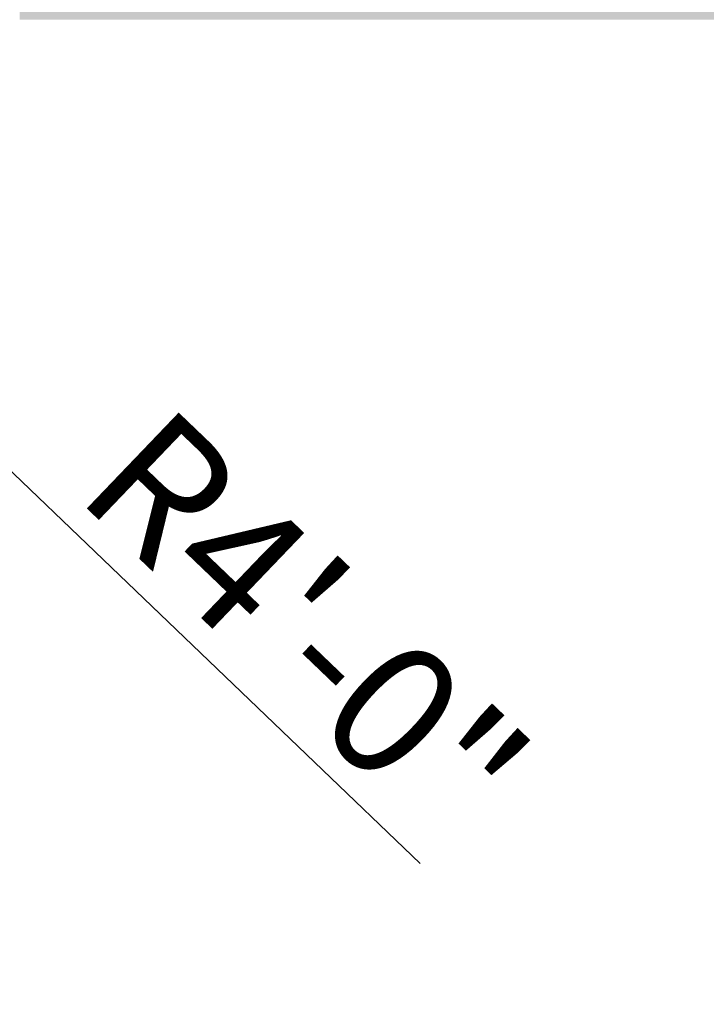
# Model space of a CAD drawing. Units: inches. Extents: x 2083 to 3317, y 1141 to 2115.
# Tile 121 of 256: x 2944 to 3006, y 1327 to 1416. Entities that reach past the tile are written whole.
import ezdxf

# ---------------------------------------------------------------- set-up
doc = ezdxf.new("R2010")
doc.units = ezdxf.units.IN
doc.layers.add('A-ANNO-DIMS', color=2, linetype='Continuous', lineweight=18)
doc.layers.add('A-WALL-PATT', color=251, linetype='Continuous', lineweight=13, true_color=0x636466)
doc.styles.get("Standard").update_dxf_attribs({"font": 'arial.ttf'})
doc.dimstyles.new('ISO-25', dxfattribs={"dimtxt": 12, "dimasz": 12, "dimexe": 1.25, "dimexo": 0.625, "dimtad": 1, "dimlunit": 3, "dimtxsty": 'Standard', "dimcen": 2.5, "dimadec": 0, "dimazin": 0, "dimtfac": 1, "dimtmove": 0, "dimatfit": 3, "dimfxl": 1, "dimarcsym": 0})

# ---------------------------------------------------------------- blocks, each defined once
blk = doc.blocks.new('*D73')
at = {"layer": 'A-ANNO-DIMS', "color": 0, "lineweight": -2, "transparency": 16777216}
for p, q in [((2895.865, 1420.763), (2930.553, 1387.52)), ((2980.105, 1340.032), (2939.217, 1379.217))]:
    blk.add_line(p, q, dxfattribs=at)
at = {"layer": 'A-ANNO-DIMS', "color": 0, "transparency": 16777216}
blk.add_solid([(2940.601, 1380.661), (2937.833, 1377.773), (2930.553, 1387.52)], dxfattribs=at)
at = {"layer": 'Defpoints', "color": 0, "transparency": 16777216}
for p in [(2895.865, 1420.763), (2930.553, 1387.52)]:
    blk.add_point(p, dxfattribs=at)
at = {"layer": 'A-ANNO-DIMS', "color": 0, "transparency": 16777216, "insert": (2968.665, 1360.348), "char_height": 12, "attachment_point": 5, "rotation": 316.21871}
blk.add_mtext('R4\'-0"', dxfattribs=at)

msp = doc.modelspace()

# ---------------------------------------------------------------- hatches: boundary and pattern name
at = {"layer": 'A-WALL-PATT'}
h = msp.add_hatch(color=256, dxfattribs=at)
h.dxf.hatch_style = 1
h.paths.add_polyline_path([(3126.96, 2020.761), (2748.96, 2020.761), (2604.96, 2020.761), (2226.96, 2020.761), (2226.96, 1702.761), (2466.96, 1702.761), (2466.96, 1582.761), (2418.96, 1582.761), (2418.96, 1477.761), (2226.96, 1477.761), (2226.96, 1263.261), (2544.96, 1263.261), (2544.96, 1411.761), (2604.96, 1411.761), (2685.96, 1411.761), (2685.96, 1420.761), (2604.96, 1420.761), (2604.96, 1573.761), (2604.96, 1702.761), (2604.96, 2011.761), (2748.96, 2011.761), (2748.96, 1702.761), (2862.96, 1702.761), (2862.96, 1621.761), (2871.96, 1621.761), (2871.96, 1702.761), (2883.96, 1702.761), (2883.96, 1706.939, -0.026459), (2883.96, 1711.761), (2757.96, 1711.761), (2757.96, 1807.761), (2787.96, 1807.761), (2787.96, 1812.261), (2757.96, 1812.261), (2757.96, 2011.761), (2877.96, 2011.761), (2877.96, 1812.261), (2847.96, 1812.261), (2847.96, 1807.761), (2889.836, 1807.761), (2889.836, 1812.261), (2882.46, 1812.261), (2882.46, 2011.761), (3117.96, 2011.761), (3117.96, 1812.261), (2937.836, 1812.261), (2937.836, 1807.761), (2995.71, 1807.761), (2995.71, 1796.118), (3000.21, 1796.118), (3000.21, 1807.761), (3117.96, 1807.761), (3117.96, 1711.761), (3000.21, 1711.761), (3000.21, 1760.118), (2998.573, 1760.118, -0.020711), (2995.71, 1760.118), (2995.71, 1711.761), (2931.96, 1711.761), (2931.96, 1702.761), (3126.96, 1702.761)])
h.paths.add_polyline_path([(2471.46, 2011.761), (2471.46, 1810.011), (2462.717, 1810.011), (2462.717, 1805.511), (2505.96, 1805.511), (2505.96, 1810.011), (2475.96, 1810.011), (2475.96, 2011.761), (2595.96, 2011.761), (2595.96, 1810.011), (2565.96, 1810.011), (2565.96, 1805.511), (2595.96, 1805.511), (2595.96, 1711.761), (2235.96, 1711.761), (2235.96, 1805.511), (2353.71, 1805.511), (2353.71, 1796.054), (2358.21, 1796.054), (2358.21, 1805.511), (2414.717, 1805.511), (2414.717, 1810.011), (2235.96, 1810.011), (2235.96, 2011.761)], flags=16)
h.paths.add_polyline_path([(2270.205, 1994.61), (2270.205, 1970.61), (2246.205, 1970.61), (2246.205, 1994.61)], flags=0)
edge = h.paths.add_edge_path(flags=0)
edge.add_ellipse((2332.027, 1899.798), major_axis=(-3.043, 3.043), ratio=0.168252, start_angle=-161.33217, end_angle=-156.30711, ccw=False)
edge.add_ellipse((2333.082, 1898.744), major_axis=(-1.055, 1.055), ratio=0.453532, start_angle=-123.37102, end_angle=-94.15911)
edge = h.paths.add_edge_path(flags=0)
edge.add_ellipse((2332.027, 1968.876), major_axis=(3.043, 3.043), ratio=0.168252, start_angle=18.66783, end_angle=23.69289)
edge.add_spline(control_points=[(2332.926, 1970.691), (2332.227, 1970.336), (2330.894, 1969.659), (2328.413, 1970.932), (2327.204, 1967.749), (2324.71, 1969.956), (2322.533, 1967.012), (2320.013, 1971.296), (2317.68, 1968.158), (2316.041, 1967.102), (2315.427, 1966.81)], knot_values=[0, 0, 0, 0, 2.267059, 4.324559, 6.685584, 8.878641, 11.121502, 14.300359, 17.755284, 19.732645, 19.732645, 19.732645, 19.732645], degree=3, periodic=0)
edge.add_ellipse((2332.027, 1968.876), major_axis=(3.043, 3.043), ratio=0.168252, start_angle=18.66783, end_angle=23.69289, ccw=False)
edge.add_ellipse((2333.082, 1969.931), major_axis=(1.055, 1.055), ratio=0.453532, start_angle=56.62898, end_angle=85.84089, ccw=False)
edge = h.paths.add_edge_path(flags=0)
edge.add_spline(control_points=[(2296.428, 1967.988), (2293.628, 1965.336), (2287.704, 1959.727), (2299.744, 1949.996), (2294.533, 1935.669), (2290.573, 1920.604), (2293.394, 1909.974), (2296.185, 1904.967)], knot_values=[0.099185, 0.099185, 0.099185, 0.099185, 0.345301, 0.619822, 0.982653, 1.386093, 1.810555, 1.810555, 1.810555, 1.810555], degree=3, periodic=0)
edge.add_spline(control_points=[(2296.185, 1904.967), (2297.384, 1902.619), (2298.001, 1901.949), (2298.553, 1901.468)], knot_values=[0.006246, 0.006246, 0.006246, 0.006246, 0.055476, 0.055476, 0.055476, 0.055476], degree=3, periodic=0)
edge.add_spline(control_points=[(2298.553, 1901.468), (2297.259, 1900.923), (2295.225, 1900.232), (2293.06, 1900.614), (2292.101, 1900.788), (2292.09, 1900.791)], knot_values=[0.312835, 0.312835, 0.312835, 0.312835, 0.40178, 0.474987, 0.475903, 0.475903, 0.475903, 0.475903], degree=3, periodic=0)
edge.add_arc((2292.794, 1904.664), 3.937, 215.4209, 259.69818, ccw=False)
edge.add_spline(control_points=[(2289.585, 1902.382), (2289.477, 1902.535), (2289.368, 1902.688), (2289.261, 1902.841)], knot_values=[0.102872, 0.102872, 0.102872, 0.102872, 0.116896, 0.116896, 0.116896, 0.116896], degree=3, periodic=0)
edge.add_spline(control_points=[(2289.261, 1902.841), (2288.687, 1902.55), (2287.64, 1902.02), (2285.881, 1901.874), (2283.853, 1901.504), (2281.72, 1899.711), (2278.467, 1899.493), (2276.157, 1901.883), (2272.259, 1899.804), (2267.778, 1901.843), (2262.244, 1900.184), (2257.415, 1901.782), (2254.318, 1900.726), (2253.178, 1900.337)], knot_values=[0, 0, 0, 0, 1.907977, 3.477176, 5.261074, 7.972851, 11.680248, 13.717921, 16.939592, 22.789562, 27.502503, 33.595215, 37.145618, 37.145618, 37.145618, 37.145618], degree=3, periodic=0)
edge.add_line((2253.178, 1900.337), (2250.244, 1902.841))
edge.add_line((2250.244, 1902.841), (2250.244, 1965.833))
edge.add_line((2250.244, 1965.833), (2253.178, 1968.337))
edge.add_spline(control_points=[(2253.178, 1968.337), (2254.318, 1967.948), (2257.415, 1966.892), (2262.244, 1968.49), (2267.778, 1966.831), (2271.527, 1968.537), (2273.876, 1967.828), (2274.207, 1967.728)], knot_values=[0, 0, 0, 0, 0.09018, 0.244935, 0.364644, 0.513233, 0.537855, 0.537855, 0.537855, 0.537855], degree=3, periodic=0)
edge.add_arc((2274.353, 1963.793), 3.937, 72.05113, 92.12795, ccw=False)
edge.add_arc((2281.297, 1985.23), 18.596, 252.05113, 288.56572)
edge.add_arc((2292.317, 1956.029), 12.646, 71.02679, 113.77822, ccw=False)
edge = h.paths.add_edge_path(flags=0)
edge.add_spline(control_points=[(2274.899, 1951.856), (2275.066, 1951.617), (2275.233, 1951.377), (2275.398, 1951.136)], knot_values=[1.409916, 1.409916, 1.409916, 1.409916, 1.43159, 1.43159, 1.43159, 1.43159], degree=3, periodic=0)
edge.add_spline(control_points=[(2275.398, 1951.136), (2275.792, 1950.562), (2276.179, 1949.984), (2276.546, 1949.397)], knot_values=[1.358238, 1.358238, 1.358238, 1.358238, 1.409916, 1.409916, 1.409916, 1.409916], degree=3, periodic=0)
edge.add_line((2276.546, 1949.397), (2277.437, 1947.862))
edge.add_spline(control_points=[(2277.437, 1947.862), (2276.304, 1945.673), (2274.64, 1942.427), (2274.632, 1938.094), (2272.799, 1930.852), (2274.356, 1943.897), (2275.948, 1947.923), (2276.546, 1949.397)], knot_values=[0.005632, 0.005632, 0.005632, 0.005632, 0.186014, 0.266002, 0.357087, 0.59639, 0.739732, 0.739732, 0.739732, 0.739732], degree=3, periodic=0)
edge.add_spline(control_points=[(2276.546, 1949.397), (2276.179, 1949.984), (2275.792, 1950.562), (2275.398, 1951.136)], knot_values=[1.358238, 1.358238, 1.358238, 1.358238, 1.409916, 1.409916, 1.409916, 1.409916], degree=3, periodic=0)
edge.add_spline(control_points=[(2275.398, 1951.136), (2274.943, 1950.08), (2274.208, 1948.025), (2273.935, 1944.851), (2272.469, 1937.627), (2273.466, 1945.696), (2274.701, 1951.059), (2274.899, 1951.856)], knot_values=[0.104364, 0.104364, 0.104364, 0.104364, 0.189636, 0.269624, 0.36071, 0.600013, 0.644622, 0.644622, 0.644622, 0.644622], degree=3, periodic=0)
h.paths.add_polyline_path([(2269.168, 1963.128, -0.357527), (2268.171, 1960.976, -0.092561), (2268.171, 1939.436, -0.357527), (2269.168, 1937.285, -0.357527), (2267.016, 1938.282, -0.164785), (2254.686, 1938.282, -0.357527), (2252.534, 1937.285, -0.357527), (2253.531, 1939.436, -0.092561), (2253.531, 1960.976, -0.357527), (2252.534, 1963.128, -0.357527), (2254.686, 1962.131, -0.164785), (2267.016, 1962.131, -0.357527)], flags=0)
h.paths.add_polyline_path([(2248.874, 1967.802), (2248.874, 1957.028), (2249.458, 1957.028), (2249.458, 1911.647), (2248.874, 1911.647), (2248.874, 1900.873), (2246.512, 1900.873, 0.197327), (2244.15, 1902.457), (2244.15, 1966.218, 0.197327), (2246.512, 1967.802)], flags=0)
h.paths.add_polyline_path([(2269.168, 1931.389, -0.357527), (2268.171, 1929.238, -0.092561), (2268.171, 1907.698, -0.357527), (2269.168, 1905.547, -0.357527), (2267.016, 1906.544, -0.164785), (2254.686, 1906.544, -0.357527), (2252.534, 1905.547, -0.357527), (2253.531, 1907.698, -0.092561), (2253.531, 1929.238, -0.357527), (2252.534, 1931.389, -0.357527), (2254.686, 1930.392, -0.164785), (2267.016, 1930.392, -0.357527)], flags=0)
edge = h.paths.add_edge_path(flags=0)
edge.add_spline(control_points=[(2276.197, 1906.724), (2276.168, 1909.029), (2276.114, 1913.372), (2270.598, 1924.925), (2273.905, 1919.013), (2275.922, 1916.262), (2275.475, 1912.402), (2277.258, 1910.381), (2276.696, 1908.225), (2276.646, 1906.813), (2276.618, 1906.008)], knot_values=[0, 0, 0, 0, 8.61026, 16.221274, 18.843057, 23.804898, 27.440828, 29.356102, 31.203478, 33.650687, 33.650687, 33.650687, 33.650687], degree=3, periodic=0)
edge.add_spline(control_points=[(2276.618, 1906.008), (2276.623, 1905.624), (2276.498, 1904.629), (2275.442, 1903.855), (2274.937, 1903.08), (2274.859, 1902.841)], knot_values=[0.156488, 0.156488, 0.156488, 0.156488, 0.184398, 0.231376, 0.250598, 0.250598, 0.250598, 0.250598], degree=3, periodic=0)
edge.add_line((2274.859, 1902.841), (2276.506, 1902.841))
edge.add_spline(control_points=[(2276.506, 1902.841), (2276.788, 1903.085), (2277.665, 1904.125), (2278.25, 1904.341), (2277.654, 1908.527), (2278.156, 1906.228), (2278.1, 1905.286), (2278.847, 1904.069), (2277.857, 1903.415), (2277.874, 1902.991), (2277.904, 1902.841)], knot_values=[0.059574, 0.059574, 0.059574, 0.059574, 0.080753, 0.103741, 0.16972, 0.176036, 0.207137, 0.240474, 0.262341, 0.27366, 0.27366, 0.27366, 0.27366], degree=3, periodic=0)
edge.add_line((2277.904, 1902.841), (2280.03, 1902.841))
edge.add_spline(control_points=[(2280.03, 1902.841), (2279.888, 1903.088), (2279.499, 1903.982), (2280.152, 1905.939), (2278.104, 1909.658), (2279.762, 1907.185), (2280.328, 1904.875), (2280.485, 1903.49), (2281.463, 1903.249), (2281.758, 1902.936), (2281.834, 1902.841)], knot_values=[0.013856, 0.013856, 0.013856, 0.013856, 0.034874, 0.088867, 0.107879, 0.126738, 0.158714, 0.193757, 0.217487, 0.226722, 0.226722, 0.226722, 0.226722], degree=3, periodic=0)
edge.add_spline(control_points=[(2281.834, 1902.841), (2281.788, 1902.827), (2281.647, 1902.783), (2281.396, 1902.859), (2281.088, 1902.985), (2280.721, 1903.061), (2280.333, 1903.026), (2280.125, 1902.899), (2280.03, 1902.841)], knot_values=[0, 0, 0, 0, 0.14413, 0.435517, 0.749276, 1.153046, 1.548371, 1.878348, 1.878348, 1.878348, 1.878348], degree=3, periodic=0)
edge.add_line((2280.03, 1902.841), (2277.904, 1902.841))
edge.add_spline(control_points=[(2277.904, 1902.841), (2277.893, 1902.796), (2277.865, 1902.68), (2277.607, 1902.687), (2277.274, 1902.801), (2276.838, 1902.62), (2276.584, 1902.789), (2276.506, 1902.841)], knot_values=[0, 0, 0, 0, 0.127189, 0.326199, 0.628009, 1.24357, 1.515331, 1.515331, 1.515331, 1.515331], degree=3, periodic=0)
edge.add_line((2276.506, 1902.841), (2274.859, 1902.841))
edge.add_spline(control_points=[(2274.859, 1902.841), (2274.814, 1902.899), (2274.725, 1903.013), (2274.493, 1903.119), (2274.244, 1902.961), (2273.937, 1903.185), (2273.614, 1902.983), (2273.408, 1902.883), (2273.322, 1902.841)], knot_values=[0, 0, 0, 0, 0.21843, 0.436957, 0.687977, 0.990379, 1.398396, 1.69185, 1.69185, 1.69185, 1.69185], degree=3, periodic=0)
edge.add_spline(control_points=[(2273.322, 1902.841), (2273.617, 1903.446), (2274.274, 1904.538), (2276.027, 1904.574), (2276.207, 1906.584), (2276.197, 1906.724)], knot_values=[0.012227, 0.012227, 0.012227, 0.012227, 0.059472, 0.106218, 0.134458, 0.134458, 0.134458, 0.134458], degree=3, periodic=0)
h.paths.add_polyline_path([(2270.776, 1897.79), (2270.776, 1873.79), (2246.776, 1873.79), (2246.776, 1897.79)], flags=0)
h.paths.add_polyline_path([(2353.71, 1760.005), (2353.71, 1760.054), (2358.21, 1760.054, -0.033729)], flags=0)
h.paths.add_polyline_path([(2321.819, 1737.529), (2341.995, 1737.529, -0.414214), (2343.203, 1736.321), (2343.203, 1721.021, -0.414214), (2341.995, 1719.813), (2321.819, 1719.813, -0.414214), (2320.611, 1721.021), (2320.611, 1736.321, -0.414214)], flags=0)
h.paths.add_polyline_path([(2324.235, 1736.321), (2339.579, 1736.321, -0.414214), (2341.995, 1733.905), (2341.995, 1725.45, -0.414214), (2339.579, 1723.034), (2333.681, 1723.034), (2333.845, 1722.045, -0.870646), (2335.425, 1721.826, -0.767327), (2333.923, 1721.423), (2331.291, 1721.423, -0.767327), (2329.788, 1721.826, -0.870646), (2331.368, 1722.045), (2331.533, 1723.034), (2324.235, 1723.034, -0.414214), (2321.819, 1725.45), (2321.819, 1733.905, -0.414214)], flags=0)
h.paths.add_polyline_path([(2570.484, 1928.615), (2589.684, 1928.615), (2590.169, 1928.615), (2590.169, 1904.993), (2570.484, 1904.993)], flags=0)
h.paths.add_polyline_path([(2574.447, 1927.264, -1), (2572.829, 1927.264, -1)], flags=0)
h.paths.add_polyline_path([(2573.09, 1926.941), (2573.925, 1927.776), (2574.148, 1927.553), (2573.313, 1926.718)], flags=0)
h.paths.add_polyline_path([(2578.779, 1919.73, -1), (2571.592, 1919.73, -1)], flags=0)
h.paths.add_polyline_path([(2578.385, 1919.73, -1), (2571.985, 1919.73, -1)], flags=0)
h.paths.add_polyline_path([(2331.596, 1729.476, -1), (2333.618, 1729.476, -1)], flags=0)
h.paths.add_polyline_path([(2578.034, 1927.264, -1), (2576.416, 1927.264, -1)], flags=0)
h.paths.add_polyline_path([(2576.689, 1927.531), (2576.912, 1927.754), (2577.747, 1926.919), (2577.524, 1926.696)], flags=0)
h.paths.add_polyline_path([(2578.139, 1909.86, -1), (2572.232, 1909.86, -1)], flags=0)
h.paths.add_polyline_path([(2577.745, 1909.86, -1), (2572.625, 1909.86, -1)], flags=0)
h.paths.add_polyline_path([(2583.798, 1927.264, -1), (2582.179, 1927.264, -1)], flags=0)
h.paths.add_polyline_path([(2582.719, 1927.754), (2583.554, 1926.919), (2583.331, 1926.696), (2582.496, 1927.531)], flags=0)
h.paths.add_polyline_path([(2582.496, 1927.531), (2582.719, 1927.754), (2583.554, 1926.919), (2583.331, 1926.696)], flags=0)
h.paths.add_polyline_path([(2587.739, 1920.53, -1), (2581.832, 1920.53, -1)], flags=0)
h.paths.add_polyline_path([(2587.345, 1920.53, -1), (2582.225, 1920.53, -1)], flags=0)
h.paths.add_polyline_path([(2587.385, 1927.264, -1), (2585.766, 1927.264, -1)], flags=0)
h.paths.add_polyline_path([(2586.082, 1926.98), (2586.917, 1927.815), (2587.14, 1927.593), (2586.305, 1926.758)], flags=0)
h.paths.add_polyline_path([(2588.379, 1910.66, -1), (2581.192, 1910.66, -1)], flags=0)
h.paths.add_polyline_path([(2587.985, 1910.66, -1), (2581.585, 1910.66, -1)], flags=0)
h.paths.add_polyline_path([(2417.168, 1729.478), (2437.344, 1729.478, -0.414214), (2438.552, 1728.27), (2438.552, 1712.969, -0.414214), (2437.344, 1711.761), (2417.168, 1711.761, -0.414214), (2415.96, 1712.969), (2415.96, 1728.27, -0.414214)], flags=0)
h.paths.add_polyline_path([(2419.584, 1728.27), (2434.928, 1728.27, -0.414214), (2437.344, 1725.854), (2437.344, 1717.398, -0.414214), (2434.928, 1714.983), (2429.029, 1714.983), (2429.194, 1713.994, -0.870646), (2430.774, 1713.775, -0.767327), (2429.271, 1713.372), (2426.64, 1713.372, -0.767327), (2425.137, 1713.775, -0.870646), (2426.717, 1713.994), (2426.882, 1714.983), (2419.584, 1714.983, -0.414214), (2417.168, 1717.398), (2417.168, 1725.854, -0.414214)], flags=0)
h.paths.add_polyline_path([(2419.584, 1728.27), (2434.928, 1728.27, -0.414214), (2437.344, 1725.854), (2437.344, 1717.398, -0.414214), (2434.928, 1714.983), (2429.029, 1714.983), (2428.358, 1719.009), (2427.553, 1719.009), (2426.882, 1714.983), (2419.584, 1714.983, -0.414214), (2417.168, 1717.398), (2417.168, 1725.854, -0.414214)], flags=0)
h.paths.add_polyline_path([(2426.944, 1721.425, -1), (2428.967, 1721.425, -1)], flags=0)
h.paths.add_polyline_path([(2475.96, 1702.761), (2595.96, 1702.761), (2595.96, 1582.761), (2475.96, 1582.761)], flags=16)
h.paths.add_polyline_path([(2427.96, 1573.761), (2595.96, 1573.761), (2595.96, 1468.761), (2595.96, 1420.761), (2384.46, 1420.761), (2384.46, 1468.761), (2427.96, 1468.761)], flags=16)
h.paths.add_polyline_path([(2379.96, 1468.761), (2379.96, 1420.761), (2235.96, 1420.761), (2235.96, 1468.761)], flags=16)
h.paths.add_polyline_path([(2317.816, 1466.696), (2337.992, 1466.696, -0.414214), (2339.2, 1465.488), (2339.2, 1450.187, -0.414214), (2337.992, 1448.979), (2317.816, 1448.979, -0.414214), (2316.608, 1450.187), (2316.608, 1465.488, -0.414214)], flags=0)
h.paths.add_polyline_path([(2320.232, 1465.488), (2335.576, 1465.488, -0.414214), (2337.992, 1463.072), (2337.992, 1454.616, -0.414214), (2335.576, 1452.2), (2329.677, 1452.2), (2329.842, 1451.212, -0.870646), (2331.422, 1450.992, -0.767327), (2329.92, 1450.59), (2327.288, 1450.59, -0.767327), (2325.785, 1450.992, -0.870646), (2327.365, 1451.212), (2327.53, 1452.2), (2320.232, 1452.2, -0.414214), (2317.816, 1454.616), (2317.816, 1463.072, -0.414214)], flags=0)
h.paths.add_polyline_path([(2320.232, 1465.488), (2335.576, 1465.488, -0.414214), (2337.992, 1463.072), (2337.992, 1454.616, -0.414214), (2335.576, 1452.2), (2329.677, 1452.2), (2329.006, 1456.227), (2328.201, 1456.227), (2327.53, 1452.2), (2320.232, 1452.2, -0.414214), (2317.816, 1454.616), (2317.816, 1463.072, -0.414214)], flags=0)
h.paths.add_polyline_path([(2327.593, 1458.643, -1), (2329.615, 1458.643, -1)], flags=0)
h.paths.add_polyline_path([(2244.412, 1433.34), (2241.921, 1433.34, -0.414214), (2240.018, 1435.244), (2240.018, 1440.953, -0.414211), (2241.921, 1442.856), (2244.412, 1442.856, -1.976472)], flags=0)
h.paths.add_polyline_path([(2245.357, 1434.398, -0.414214), (2245.357, 1441.799, -2.144098)], flags=0)
h.paths.add_polyline_path([(2535.96, 1416.261), (2535.96, 1272.261), (2235.96, 1272.261), (2235.96, 1416.261)], flags=16)
h.paths.add_polyline_path([(2260.12, 1384.293), (2260.12, 1362.039), (2237.865, 1362.039), (2237.865, 1384.293)], flags=0)
edge = h.paths.add_edge_path(flags=0)
edge.add_line((2318.252, 1362.093), (2318.146, 1362.001))
edge.add_ellipse((2317.445, 1360.431), major_axis=(2.822, 2.822), ratio=0.168252, start_angle=18.66783, end_angle=20.94813, ccw=False)
edge.add_ellipse((2318.423, 1361.409), major_axis=(0.978, 0.978), ratio=0.453532, start_angle=56.62898, end_angle=70.2262, ccw=False)
edge = h.paths.add_edge_path(flags=0)
edge.add_line((2319.107, 1295.571), (2319.015, 1295.677))
edge.add_ellipse((2317.445, 1296.378), major_axis=(-2.822, 2.822), ratio=0.168252, start_angle=-161.33217, end_angle=-159.05187, ccw=False)
edge.add_ellipse((2318.423, 1295.4), major_axis=(-0.978, 0.978), ratio=0.453532, start_angle=-123.37102, end_angle=-109.7738)
edge = h.paths.add_edge_path(flags=0)
edge.add_spline(control_points=[(2284.21, 1301.17), (2284.581, 1300.445), (2284.891, 1299.892), (2285.16, 1299.461)], knot_values=[0.039066, 0.039066, 0.039066, 0.039066, 0.055476, 0.055476, 0.055476, 0.055476], degree=3, periodic=0)
edge.add_line((2285.16, 1299.461), (2284.21, 1301.17))
edge = h.paths.add_edge_path(flags=0)
edge.add_line((2280.412, 1297.298), (2283.37, 1297.036))
edge.add_line((2283.37, 1297.036), (2286.406, 1297.926))
edge.add_spline(control_points=[(2286.406, 1297.926), (2285.305, 1297.463), (2284.345, 1297.129), (2283.37, 1297.036)], knot_values=[0.394369, 0.394369, 0.394369, 0.394369, 0.475903, 0.475903, 0.475903, 0.475903], degree=3, periodic=0)
edge.add_spline(control_points=[(2283.37, 1297.036), (2283.281, 1297.028), (2282.316, 1296.957), (2281.313, 1297.134), (2280.423, 1297.296), (2280.412, 1297.298)], knot_values=[0.312835, 0.312835, 0.312835, 0.312835, 0.320246, 0.393453, 0.394369, 0.394369, 0.394369, 0.394369], degree=3, periodic=0)
edge = h.paths.add_edge_path(flags=0)
edge.add_line((2284.436, 1359.607), (2280.446, 1355.328))
edge.add_line((2280.446, 1355.328), (2279.58, 1351.018))
edge.add_line((2279.58, 1351.018), (2282.413, 1346.58))
edge.add_spline(control_points=[(2282.413, 1346.58), (2283.153, 1345.589), (2284.253, 1344.029), (2284.801, 1342.387), (2284.935, 1341.806)], knot_values=[1.240098, 1.240098, 1.240098, 1.240098, 1.332892, 1.382712, 1.382712, 1.382712, 1.382712], degree=3, periodic=0)
edge.add_spline(control_points=[(2284.935, 1341.806), (2285.319, 1340.141), (2285.233, 1338.409), (2284.91, 1336.654)], knot_values=[1.097484, 1.097484, 1.097484, 1.097484, 1.240098, 1.240098, 1.240098, 1.240098], degree=3, periodic=0)
edge.add_spline(control_points=[(2284.91, 1336.654), (2284.587, 1334.899), (2284.027, 1333.12), (2283.463, 1331.361)], knot_values=[0.95487, 0.95487, 0.95487, 0.95487, 1.097484, 1.097484, 1.097484, 1.097484], degree=3, periodic=0)
edge.add_line((2283.463, 1331.361), (2281.89, 1326.153))
edge.add_line((2281.89, 1326.153), (2280.756, 1321.056))
edge.add_line((2280.756, 1321.056), (2280.299, 1316.002))
edge.add_line((2280.299, 1316.002), (2280.716, 1310.95))
edge.add_line((2280.716, 1310.95), (2282.028, 1305.972))
edge.add_line((2282.028, 1305.972), (2284.21, 1301.17))
edge.add_spline(control_points=[(2284.21, 1301.17), (2283.341, 1302.73), (2282.612, 1304.336), (2282.028, 1305.972)], knot_values=[0.099185, 0.099185, 0.099185, 0.099185, 0.241799, 0.241799, 0.241799, 0.241799], degree=3, periodic=0)
edge.add_spline(control_points=[(2282.028, 1305.972), (2281.444, 1307.608), (2281.005, 1309.273), (2280.716, 1310.95)], knot_values=[0.241799, 0.241799, 0.241799, 0.241799, 0.384413, 0.384413, 0.384413, 0.384413], degree=3, periodic=0)
edge.add_spline(control_points=[(2280.716, 1310.95), (2280.433, 1312.588), (2280.289, 1314.277), (2280.299, 1315.962), (2280.299, 1316.002)], knot_values=[0.384413, 0.384413, 0.384413, 0.384413, 0.523647, 0.527028, 0.527028, 0.527028, 0.527028], degree=3, periodic=0)
edge.add_spline(control_points=[(2280.299, 1316.002), (2280.312, 1317.687), (2280.478, 1319.368), (2280.756, 1321.056)], knot_values=[0.527028, 0.527028, 0.527028, 0.527028, 0.669642, 0.669642, 0.669642, 0.669642], degree=3, periodic=0)
edge.add_spline(control_points=[(2280.756, 1321.056), (2281.035, 1322.744), (2281.426, 1324.44), (2281.89, 1326.153)], knot_values=[0.669642, 0.669642, 0.669642, 0.669642, 0.812256, 0.812256, 0.812256, 0.812256], degree=3, periodic=0)
edge.add_spline(control_points=[(2281.89, 1326.153), (2282.264, 1327.533), (2282.788, 1329.262), (2283.353, 1331.018), (2283.463, 1331.361)], knot_values=[0.812256, 0.812256, 0.812256, 0.812256, 0.927087, 0.95487, 0.95487, 0.95487, 0.95487], degree=3, periodic=0)
edge.add_line((2283.463, 1331.361), (2284.91, 1336.654))
edge.add_line((2284.91, 1336.654), (2284.935, 1341.806))
edge.add_line((2284.935, 1341.806), (2282.413, 1346.58))
edge.add_spline(control_points=[(2282.413, 1346.58), (2281.275, 1348.104), (2280.078, 1349.57), (2279.58, 1351.018)], knot_values=[1.382712, 1.382712, 1.382712, 1.382712, 1.525326, 1.525326, 1.525326, 1.525326], degree=3, periodic=0)
edge.add_spline(control_points=[(2279.58, 1351.018), (2279.443, 1351.415), (2279.136, 1352.857), (2279.735, 1354.29), (2280.446, 1355.328)], knot_values=[1.525326, 1.525326, 1.525326, 1.525326, 1.564439, 1.667941, 1.667941, 1.667941, 1.667941], degree=3, periodic=0)
edge.add_spline(control_points=[(2280.446, 1355.328), (2281.426, 1356.758), (2282.931, 1358.183), (2284.436, 1359.607)], knot_values=[1.667941, 1.667941, 1.667941, 1.667941, 1.810555, 1.810555, 1.810555, 1.810555], degree=3, periodic=0)
edge.add_arc((2280.623, 1348.518), 11.726, 71.02679, 113.77822)
edge.add_arc((2270.405, 1375.595), 17.244, 252.05113, 288.56572, ccw=False)
edge.add_arc((2263.966, 1355.718), 3.651, 72.05113, 92.12795)
edge.add_arc((2263.966, 1355.718), 3.651, 92.12795, 177.98513)
edge.add_spline(control_points=[(2260.318, 1355.846), (2260.26, 1354.221), (2260.551, 1350.187), (2262.999, 1346.766), (2264.473, 1344.649)], knot_values=[1.43159, 1.43159, 1.43159, 1.43159, 1.564144, 1.770695, 1.770695, 1.770695, 1.770695], degree=3, periodic=0)
edge.add_line((2264.473, 1344.649), (2264.936, 1343.983))
edge.add_spline(control_points=[(2263.801, 1340.248), (2263.843, 1340.514), (2264.067, 1341.756), (2264.513, 1343.002), (2264.935, 1343.981)], knot_values=[0.53657, 0.53657, 0.53657, 0.53657, 0.559349, 0.644622, 0.644622, 0.644622, 0.644622], degree=3, periodic=0)
edge.add_spline(control_points=[(2264.935, 1343.981), (2265.118, 1343.715), (2265.299, 1343.448), (2265.477, 1343.179)], knot_values=[1.384077, 1.384077, 1.384077, 1.384077, 1.409916, 1.409916, 1.409916, 1.409916], degree=3, periodic=0)
edge.add_spline(control_points=[(2265.477, 1343.179), (2265.655, 1342.911), (2265.829, 1342.641), (2265.999, 1342.369)], knot_values=[1.358238, 1.358238, 1.358238, 1.358238, 1.384077, 1.384077, 1.384077, 1.384077], degree=3, periodic=0)
edge.add_line((2265.999, 1342.369), (2266.826, 1340.946))
edge.add_spline(control_points=[(2266.826, 1340.946), (2268.894, 1337.09), (2271.398, 1325.843), (2270.516, 1310.569), (2275.919, 1301.861), (2277.79, 1299.199)], knot_values=[0.116896, 0.116896, 0.116896, 0.116896, 0.472987, 1.050969, 1.313793, 1.313793, 1.313793, 1.313793], degree=3, periodic=0)
edge.add_spline(control_points=[(2277.79, 1299.199), (2277.839, 1299.128), (2277.889, 1299.057), (2277.94, 1298.987)], knot_values=[0.109884, 0.109884, 0.109884, 0.109884, 0.116896, 0.116896, 0.116896, 0.116896], degree=3, periodic=0)
edge.add_line((2277.94, 1298.987), (2277.789, 1299.199))
edge.add_spline(control_points=[(2277.789, 1299.199), (2277.257, 1298.929), (2276.286, 1298.438), (2275.039, 1298.334), (2274.383, 1298.239), (2274.215, 1298.209)], knot_values=[33.12187, 33.12187, 33.12187, 33.12187, 35.029056, 36.598255, 37.144827, 37.144827, 37.144827, 37.144827], degree=3, periodic=0)
edge.add_line((2274.215, 1298.209), (2273.073, 1297.893))
edge.add_spline(control_points=[(2273.073, 1297.893), (2272.323, 1297.58), (2271.039, 1296.511), (2269.248, 1296.226), (2268.423, 1296.375)], knot_values=[26.532584, 26.532584, 26.532584, 26.532584, 29.198919, 31.839101, 31.839101, 31.839101, 31.839101], degree=3, periodic=0)
edge.add_line((2268.423, 1296.375), (2263.879, 1297.458))
edge.add_spline(control_points=[(2263.879, 1297.458), (2263.556, 1297.359), (2261.86, 1296.839), (2260.239, 1297.282), (2258.933, 1297.516)], knot_values=[15.919551, 15.919551, 15.919551, 15.919551, 16.939592, 21.226067, 21.226067, 21.226067, 21.226067], degree=3, periodic=0)
edge.add_line((2258.933, 1297.516), (2254.055, 1297.329))
edge.add_spline(control_points=[(2254.055, 1297.329), (2253.756, 1297.296), (2252.114, 1297.165), (2250.462, 1297.544), (2249.13, 1297.668)], knot_values=[5.306517, 5.306517, 5.306517, 5.306517, 6.276435, 10.613034, 10.613034, 10.613034, 10.613034], degree=3, periodic=0)
edge.add_line((2249.13, 1297.668), (2244.332, 1296.878))
edge.add_line((2244.332, 1296.878), (2241.611, 1299.199))
edge.add_line((2241.611, 1299.199), (2241.611, 1357.609))
edge.add_line((2241.611, 1357.609), (2244.332, 1359.931))
edge.add_line((2244.332, 1359.931), (2252.729, 1359.543))
edge.add_spline(control_points=[(2252.729, 1359.543), (2252.871, 1359.546), (2253.306, 1359.548), (2253.74, 1359.514), (2254.032, 1359.482)], knot_values=[0.233291, 0.233291, 0.233291, 0.233291, 0.244935, 0.268927, 0.268927, 0.268927, 0.268927], degree=3, periodic=0)
edge.add_line((2254.032, 1359.482), (2259.587, 1359.416))
edge.add_spline(control_points=[(2259.587, 1359.416), (2260.677, 1359.629), (2262.073, 1359.897), (2263.524, 1359.459), (2263.83, 1359.366)], knot_values=[0.422516, 0.422516, 0.422516, 0.422516, 0.513233, 0.537855, 0.537855, 0.537855, 0.537855], degree=3, periodic=0)
edge.add_arc((2263.966, 1355.718), 3.651, 72.05113, 92.12795, ccw=False)
edge.add_arc((2270.405, 1375.595), 17.244, 252.05113, 288.56572)
edge.add_arc((2280.623, 1348.518), 11.726, 71.02679, 113.77822, ccw=False)
h.paths.add_polyline_path([(2240.341, 1359.435), (2240.341, 1349.444), (2240.882, 1349.444), (2240.882, 1307.365), (2240.341, 1307.365), (2240.341, 1297.374), (2238.15, 1297.374, 0.197327), (2235.96, 1298.843), (2235.96, 1357.966, 0.197327), (2238.15, 1359.435)], flags=0)
h.paths.add_polyline_path([(2259.158, 1355.101, -0.357527), (2258.233, 1353.106, -0.092561), (2258.233, 1333.133, -0.357527), (2259.158, 1331.138, -0.357527), (2257.163, 1332.062, -0.164785), (2245.729, 1332.062, -0.357527), (2243.735, 1331.138, -0.357527), (2244.659, 1333.133, -0.092561), (2244.659, 1353.106, -0.357527), (2243.735, 1355.101, -0.357527), (2245.729, 1354.176, -0.164785), (2257.163, 1354.176, -0.357527)], flags=0)
edge = h.paths.add_edge_path(flags=0)
edge.add_line((2265.999, 1342.369), (2266.826, 1340.946))
edge.add_line((2266.826, 1340.946), (2265.308, 1337.814))
edge.add_line((2265.308, 1337.814), (2264.358, 1334.653))
edge.add_line((2264.358, 1334.653), (2264.262, 1333.8))
edge.add_spline(control_points=[(2264.262, 1333.8), (2264.208, 1333.187), (2264.162, 1332.366), (2264.007, 1331.414), (2263.969, 1331.202)], knot_values=[0.464444, 0.464444, 0.464444, 0.464444, 0.516691, 0.531608, 0.531608, 0.531608, 0.531608], degree=3, periodic=0)
edge.add_spline(control_points=[(2263.969, 1331.202), (2263.775, 1330.119), (2263.424, 1328.791), (2263.257, 1328.531), (2263.234, 1328.515)], knot_values=[0.372682, 0.372682, 0.372682, 0.372682, 0.44885, 0.464444, 0.464444, 0.464444, 0.464444], degree=3, periodic=0)
edge.add_spline(control_points=[(2263.234, 1328.515), (2263.096, 1328.42), (2263.131, 1329.301), (2263.275, 1330.616)], knot_values=[0.280919, 0.280919, 0.280919, 0.280919, 0.372682, 0.372682, 0.372682, 0.372682], degree=3, periodic=0)
edge.add_spline(control_points=[(2263.275, 1330.616), (2263.419, 1331.93), (2263.672, 1333.677), (2263.97, 1335.315)], knot_values=[0.189157, 0.189157, 0.189157, 0.189157, 0.280919, 0.280919, 0.280919, 0.280919], degree=3, periodic=0)
edge.add_spline(control_points=[(2263.97, 1335.315), (2264.1, 1336.032), (2264.419, 1337.622), (2264.755, 1338.864), (2264.947, 1339.491)], knot_values=[0.097394, 0.097394, 0.097394, 0.097394, 0.137578, 0.189157, 0.189157, 0.189157, 0.189157], degree=3, periodic=0)
edge.add_spline(control_points=[(2264.947, 1339.491), (2265.29, 1340.606), (2265.644, 1341.494), (2265.999, 1342.369)], knot_values=[0.005632, 0.005632, 0.005632, 0.005632, 0.097394, 0.097394, 0.097394, 0.097394], degree=3, periodic=0)
h.paths.add_polyline_path([(2259.158, 1325.671, -0.357527), (2258.233, 1323.676, -0.092561), (2258.233, 1303.703, -0.357527), (2259.158, 1301.708, -0.357527), (2257.163, 1302.633, -0.164785), (2245.729, 1302.633, -0.357527), (2243.735, 1301.708, -0.357527), (2244.659, 1303.703, -0.092561), (2244.659, 1323.676, -0.357527), (2243.735, 1325.671, -0.357527), (2245.729, 1324.747, -0.164785), (2257.163, 1324.747, -0.357527)], flags=0)
edge = h.paths.add_edge_path(flags=0)
edge.add_spline(control_points=[(2261.709, 1317.311), (2261.679, 1317.418), (2261.762, 1317.389), (2262.491, 1316.09), (2262.962, 1315.301)], knot_values=[14.955861, 14.955861, 14.955861, 14.955861, 16.221274, 18.694826, 18.694826, 18.694826, 18.694826], degree=3, periodic=0)
edge.add_spline(control_points=[(2262.962, 1315.301), (2262.99, 1315.254), (2263.702, 1314.067), (2264.349, 1313.127), (2264.73, 1312.164)], knot_values=[18.694826, 18.694826, 18.694826, 18.694826, 18.843057, 22.433791, 22.433791, 22.433791, 22.433791], degree=3, periodic=0)
edge.add_spline(control_points=[(2264.73, 1312.164), (2264.876, 1311.796), (2265.177, 1310.77), (2265.143, 1309.559), (2265.248, 1308.824)], knot_values=[22.433791, 22.433791, 22.433791, 22.433791, 23.804898, 26.172756, 26.172756, 26.172756, 26.172756], degree=3, periodic=0)
edge.add_line((2265.248, 1308.824), (2265.851, 1307.172))
edge.add_spline(control_points=[(2265.851, 1307.172), (2266.065, 1306.822), (2266.384, 1306.332), (2266.424, 1305.781), (2266.42, 1305.611)], knot_values=[28.062562, 28.062562, 28.062562, 28.062562, 29.356102, 29.911721, 29.911721, 29.911721, 29.911721], degree=3, periodic=0)
edge.add_spline(control_points=[(2266.42, 1305.611), (2266.416, 1305.433), (2266.394, 1305.25), (2266.365, 1305.066)], knot_values=[29.911721, 29.911721, 29.911721, 29.911721, 30.497837, 30.497837, 30.497837, 30.497837], degree=3, periodic=0)
edge.add_line((2266.365, 1305.066), (2266.066, 1302.136))
edge.add_spline(control_points=[(2266.066, 1302.136), (2266.071, 1301.78), (2265.998, 1301.2), (2265.663, 1300.759), (2265.509, 1300.586)], knot_values=[0.156488, 0.156488, 0.156488, 0.156488, 0.184398, 0.203543, 0.203543, 0.203543, 0.203543], degree=3, periodic=0)
edge.add_line((2265.509, 1300.586), (2264.435, 1299.199))
edge.add_line((2264.435, 1299.199), (2265.962, 1299.199))
edge.add_line((2265.962, 1299.199), (2267.336, 1301.175))
edge.add_line((2267.336, 1301.175), (2267.312, 1301.986))
edge.add_spline(control_points=[(2267.312, 1301.986), (2267.261, 1302.862), (2267.16, 1303.737), (2267.271, 1303.326)], knot_values=[0.126229, 0.126229, 0.126229, 0.126229, 0.166617, 0.166617, 0.166617, 0.166617], degree=3, periodic=0)
edge.add_spline(control_points=[(2267.271, 1303.326), (2267.28, 1303.294), (2267.31, 1303.175), (2267.373, 1302.884), (2267.406, 1302.683), (2267.418, 1302.601)], knot_values=[0.166617, 0.166617, 0.166617, 0.166617, 0.16972, 0.176036, 0.180765, 0.180765, 0.180765, 0.180765], degree=3, periodic=0)
edge.add_spline(control_points=[(2267.744, 1300.988), (2267.688, 1301.151), (2267.481, 1301.657), (2267.484, 1302.145), (2267.418, 1302.601)], knot_values=[0.180765, 0.180765, 0.180765, 0.180765, 0.193767, 0.220139, 0.220139, 0.220139, 0.220139], degree=3, periodic=0)
edge.add_line((2267.418, 1302.601), (2267.744, 1300.988))
edge.add_spline(control_points=[(2267.744, 1300.988), (2267.832, 1300.732), (2267.932, 1300.31), (2267.555, 1299.975), (2267.429, 1299.829)], knot_values=[0.220139, 0.220139, 0.220139, 0.220139, 0.240474, 0.25489, 0.25489, 0.25489, 0.25489], degree=3, periodic=0)
edge.add_line((2267.429, 1299.829), (2267.258, 1299.199))
edge.add_line((2267.258, 1299.199), (2269.23, 1299.199))
edge.add_spline(control_points=[(2269.23, 1299.199), (2269.099, 1299.429), (2268.843, 1300.016), (2269.012, 1300.916), (2268.947, 1301.661)], knot_values=[0.013856, 0.013856, 0.013856, 0.013856, 0.034874, 0.067073, 0.067073, 0.067073, 0.067073], degree=3, periodic=0)
edge.add_line((2268.947, 1301.661), (2268.432, 1303.603))
edge.add_spline(control_points=[(2268.432, 1303.603), (2268.176, 1304.192), (2267.596, 1305.251), (2268.041, 1304.623), (2268.251, 1304.282)], knot_values=[0.090155, 0.090155, 0.090155, 0.090155, 0.107879, 0.120289, 0.120289, 0.120289, 0.120289], degree=3, periodic=0)
edge.add_spline(control_points=[(2268.251, 1304.282), (2268.361, 1304.105), (2269.058, 1302.918), (2269.383, 1301.59), (2269.521, 1300.776), (2269.575, 1300.556)], knot_values=[0.120289, 0.120289, 0.120289, 0.120289, 0.126738, 0.158714, 0.173506, 0.173506, 0.173506, 0.173506], degree=3, periodic=0)
edge.add_line((2269.575, 1300.556), (2270.686, 1299.421))
edge.add_spline(control_points=[(2270.686, 1299.421), (2270.767, 1299.357), (2270.838, 1299.281), (2270.903, 1299.199)], knot_values=[0.21816, 0.21816, 0.21816, 0.21816, 0.226722, 0.226722, 0.226722, 0.226722], degree=3, periodic=0)
edge.add_line((2270.937, 1299.193), (2270.903, 1299.199))
edge.add_spline(control_points=[(2270.903, 1299.199), (2270.86, 1299.186), (2270.73, 1299.146), (2270.496, 1299.216), (2270.272, 1299.308), (2270.121, 1299.348), (2270.063, 1299.36)], knot_values=[0.939174, 0.939174, 0.939174, 0.939174, 1.083304, 1.374691, 1.68845, 1.878348, 1.878348, 1.878348, 1.878348], degree=3, periodic=0)
edge.add_line((2270.063, 1299.36), (2269.23, 1299.199))
edge.add_line((2269.23, 1299.199), (2267.258, 1299.199))
edge.add_spline(control_points=[(2267.258, 1299.199), (2267.248, 1299.157), (2267.223, 1299.05), (2266.984, 1299.057), (2266.809, 1299.116), (2266.677, 1299.109), (2266.637, 1299.105)], knot_values=[0.757665, 0.757665, 0.757665, 0.757665, 0.884854, 1.083864, 1.385675, 1.515331, 1.515331, 1.515331, 1.515331], degree=3, periodic=0)
edge.add_spline(control_points=[(2266.637, 1299.105), (2266.485, 1299.089), (2266.236, 1299.017), (2266.035, 1299.151), (2265.962, 1299.199)], knot_values=[0, 0, 0, 0, 0.485905, 0.757665, 0.757665, 0.757665, 0.757665], degree=3, periodic=0)
edge.add_line((2265.962, 1299.199), (2264.435, 1299.199))
edge.add_line((2264.435, 1299.199), (2263.858, 1299.367))
edge.add_spline(control_points=[(2263.858, 1299.367), (2263.819, 1299.371), (2263.78, 1299.386), (2263.74, 1299.402)], knot_values=[0.845925, 0.845925, 0.845925, 0.845925, 0.978627, 0.978627, 0.978627, 0.978627], degree=3, periodic=0)
edge.add_line((2263.722, 1299.396), (2263.01, 1299.199))
edge.add_spline(control_points=[(2263.01, 1299.199), (2263.246, 1299.683), (2263.506, 1300.128), (2263.873, 1300.408)], knot_values=[0.012227, 0.012227, 0.012227, 0.012227, 0.052971, 0.052971, 0.052971, 0.052971], degree=3, periodic=0)
edge.add_spline(control_points=[(2263.873, 1300.408), (2263.932, 1300.453), (2264.084, 1300.553), (2264.255, 1300.624), (2264.36, 1300.665)], knot_values=[0.052971, 0.052971, 0.052971, 0.052971, 0.059472, 0.069086, 0.069086, 0.069086, 0.069086], degree=3, periodic=0)
edge.add_line((2264.36, 1300.665), (2265.142, 1301.078))
edge.add_line((2265.142, 1301.078), (2265.676, 1302.8))
edge.add_line((2265.676, 1302.8), (2265.541, 1305.704))
edge.add_line((2265.541, 1305.704), (2264.803, 1309.328))
edge.add_line((2264.803, 1309.328), (2263.041, 1314.092))
edge.add_spline(control_points=[(2263.041, 1314.092), (2262.384, 1315.671), (2261.796, 1316.998), (2261.709, 1317.311)], knot_values=[11.216896, 11.216896, 11.216896, 11.216896, 14.955861, 14.955861, 14.955861, 14.955861], degree=3, periodic=0)
h.paths.add_polyline_path([(2871.96, 1416.261), (2895.91, 1416.261), (2895.91, 1420.761), (2871.96, 1420.761), (2871.96, 1501.761), (2862.96, 1501.761), (2862.96, 1420.761), (2805.96, 1420.761), (2805.96, 1411.761), (2862.96, 1411.761), (2862.96, 1263.261), (3126.96, 1263.261), (3126.96, 1411.761), (3126.96, 1486.761), (2943.96, 1486.761), (2943.96, 1477.761), (2967.86, 1477.761), (2967.86, 1420.761), (2943.91, 1420.761), (2943.91, 1416.261), (3117.96, 1416.261), (3117.96, 1420.761), (2972.36, 1420.761), (2972.36, 1477.761), (3117.96, 1477.761), (3117.96, 1420.761), (3117.96, 1272.261), (2871.96, 1272.261)], flags=0)
h.paths.add_polyline_path([(2457.126, 1485.943), (2527.603, 1485.943), (2527.603, 1537.636), (2457.126, 1537.636)], flags=8)
h.paths.add_polyline_path([(2481.005, 1609.982), (2590.766, 1609.982), (2590.766, 1682.003), (2481.005, 1682.003)], flags=8)
h.paths.add_polyline_path([(2483.085, 1729.127), (2553.562, 1729.127), (2553.562, 1780.82), (2483.085, 1780.82)], flags=8)
h = msp.add_hatch(color=256, dxfattribs=at)
h.dxf.hatch_style = 1
h.paths.add_polyline_path([(3126.96, 1486.761), (2943.96, 1486.761), (2943.96, 1477.761), (2967.86, 1477.761), (2967.86, 1420.761), (2943.91, 1420.761), (2943.91, 1416.261), (3117.96, 1416.261), (3117.96, 1420.761), (2972.36, 1420.761), (2972.36, 1477.761), (3117.96, 1477.761), (3117.96, 1420.761), (3117.96, 1272.261), (2871.96, 1272.261), (2871.96, 1416.261), (2895.91, 1416.261), (2895.91, 1420.761), (2871.96, 1420.761), (2871.96, 1501.761), (2862.96, 1501.761), (2862.96, 1420.761), (2805.96, 1420.761), (2805.96, 1411.761), (2862.96, 1411.761), (2862.96, 1263.261), (3126.96, 1263.261), (3126.96, 1411.761)])

# ---------------------------------------------------------------- dimensions: what is measured, and where the dimension line sits
at = {"layer": 'A-ANNO-DIMS'}
dim = msp.add_radius_dim(center=(2895.865, 1420.763), mpoint=(2930.553, 1387.52), dimstyle='ISO-25', override={"dimdec": 1, "dimlfac": 1, "dimrnd": 0, "dimzin": 1, "dimdsep": 46, "dimlunit": 4, "dimfrac": 2}, dxfattribs=at)
dim.commit()
dim.dimension.update_dxf_attribs({"geometry": '*D73', "text_midpoint": (2968.665, 1360.348)})

doc.saveas('drawing.dxf')
